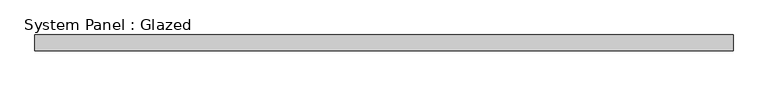
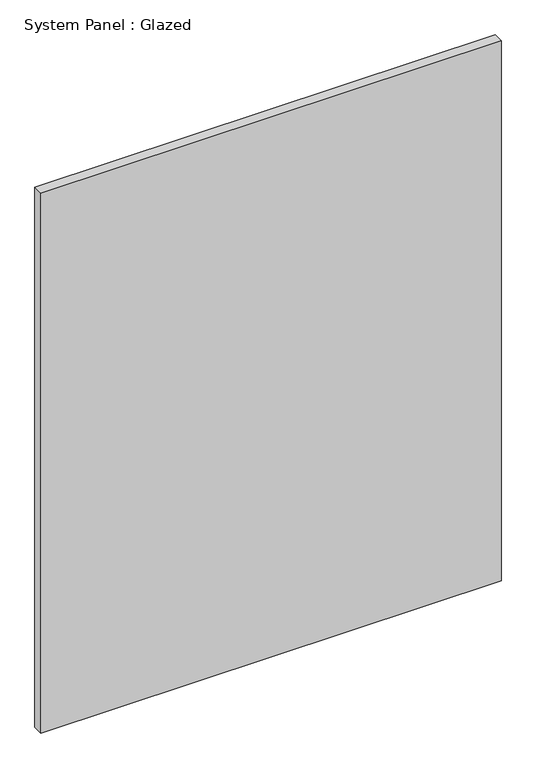
"""IFC4 building model written with IfcOpenShell, lengths in millimetres: plate geometry, System Panel : Glazed."""

from ifc_helpers import new_model, si_unit, origin, origin_with_axes, place, context, project, spatial, polyline, outline, extrude, source, transform, mapped, element, save


def system_panel_glazed_53f2b764(model_context):
    return source(origin(), model_context, "Body", "SweptSolid", [
        extrude(outline(polyline([(561.975, 19.05), (-561.975, 19.05), (-561.975, 44.45), (561.975, 44.45), (561.975, 19.05)])), origin_with_axes(), (0.0, 0.0, 1.0), 1394.1896321),
    ])


if __name__ == "__main__":
    model = new_model("IFC4")
    model_context = context("Model", 3, world=origin())
    ifc_project = project(units=[si_unit("LENGTHUNIT", "METRE", prefix="MILLI")], contexts=[model_context])
    site = spatial("IfcSite", under=ifc_project)
    building = spatial("IfcBuilding", under=site)
    placement = place(None, origin())
    system_panel_glazed_shape = system_panel_glazed_53f2b764(model_context)
    element("IfcPlate", 1, ObjectType="System Panel : Glazed", at=placement, inside=building, context=model_context, shape_type="MappedRepresentation", body=[
        mapped(system_panel_glazed_shape, transform((0.0, 0.0, 0.0), x_axis=(1.0, 0.0, 0.0), y_axis=(0.0, 1.0, 0.0), z_axis=(0.0, 0.0, 1.0))),
    ])
    save(model, "model.ifc")

# Revit data of these elements
# Type "System Panel : Glazed"
#   Construction Type Id = "GSP4R"
#   Analytic Construction = "1/8 in Pilkington single glazing"
#   Visual Light Transmittance = 0.9
#   Solar Heat Gain Coefficient = 0.86
#   Heat Transfer Coefficient (U) = 1.18115 BTU/(h·ft²·°F)
#   Define Thermal Properties by = 1
# Element 1 (IfcPlate, "System Panel : Glazed")
#   Materials on its faces: "Glass"
# Materials
#   "Glass": class "Glass", colour RGB 0 128 192, transparency 0.75, Description = "Soda Lime Glass", Cost = 0
